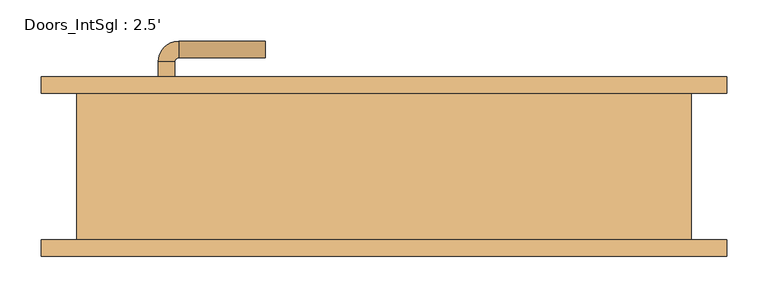
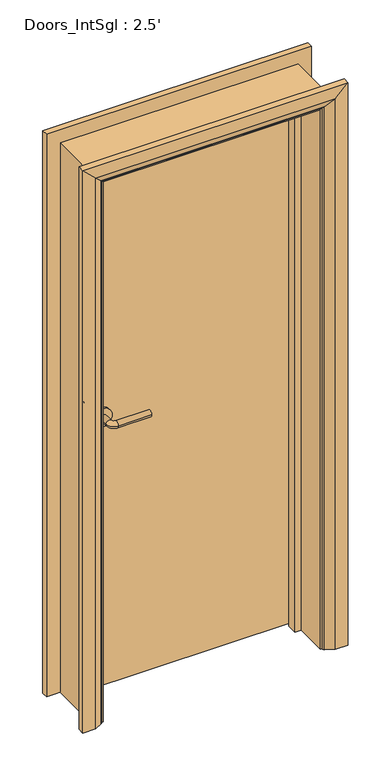
"""IFC4 building model written with IfcOpenShell, lengths in millimetres: door geometry, Doors_IntSgl : 2.5'."""

from ifc_helpers import new_model, si_unit, point, frame, frame_2d, origin, place, context, project, spatial, polyline, circle_curve, ellipse_curve, trimmed, segment, composite_curve, outline, extrude, faceted_brep, source, transform, mapped, element, save
from ifc_brep_helpers import plane_surface, cylinder_surface, revolved_surface, advanced_brep


def doors_intsgl_2_5_ea0f4f48(model_context):
    return source(origin(), model_context, "Body", "SolidModel", [
        advanced_brep(
        [(-274.0, 42.9, 900.0), (-254.0, 42.9, 900.0), (-254.0, 12.9, 900.0), (-274.0, 12.9, 900.0), (-249.0, 7.9, 900.0), (-249.0, -12.1, 900.0), (-144.0, -12.1, 900.0), (-144.0, 7.9, 900.0)],
        [
            (0, 1, circle_curve(frame((-264.0, 42.9, 900.0), z_axis=(0.0, 1.0, 0.0), x_axis=(1.0, 0.0, 0.0)), 10.0)),
            (1, 0, circle_curve(frame((-264.0, 42.9, 900.0), z_axis=(0.0, 1.0, 0.0), x_axis=(1.0, 0.0, 0.0)), 10.0)),
            (1, 2),
            (2, 3, circle_curve(frame((-264.0, 12.9, 900.0), z_axis=(0.0, 1.0, 0.0), x_axis=(1.0, 0.0, 0.0)), 10.0)),
            (3, 0),
            (3, 2, circle_curve(frame((-264.0, 12.9, 900.0), z_axis=(0.0, 1.0, 0.0), x_axis=(1.0, 0.0, 0.0)), 10.0)),
            (4, 5, circle_curve(frame((-249.0, -2.1, 900.0), z_axis=(-1.0, 0.0, 0.0), x_axis=(0.0, 1.0, 0.0)), 10.0)),
            (5, 3, circle_curve(frame((-249.0, 12.9, 900.0), z_axis=(0.0, 0.0, -1.0), x_axis=(-1.0, 0.0, 0.0)), 25.0)),
            (2, 4, circle_curve(frame((-249.0, 12.9, 900.0), z_axis=(0.0, 0.0, 1.0), x_axis=(-1.0, 0.0, 0.0)), 5.0)),
            (5, 4, circle_curve(frame((-249.0, -2.1, 900.0), z_axis=(-1.0, 0.0, 0.0), x_axis=(0.0, 1.0, 0.0)), 10.0)),
            (6, 7, circle_curve(frame((-144.0, -2.1, 900.0), z_axis=(1.0, 0.0, 0.0), x_axis=(0.0, 1.0, 0.0)), 10.0)),
            (7, 6, circle_curve(frame((-144.0, -2.1, 900.0), z_axis=(1.0, 0.0, 0.0), x_axis=(0.0, 1.0, 0.0)), 10.0)),
            (4, 7),
            (6, 5),
        ],
        [
            plane_surface(frame((-264.0, 42.9, 900.0), z_axis=(0.0, 1.0, 0.0), x_axis=(0.0, 0.0, 1.0))),
            cylinder_surface(frame((-264.0, 42.9, 900.0), z_axis=(0.0, 1.0, 0.0), x_axis=(1.0, 0.0, 0.0)), 10.0),
            revolved_surface(trimmed(ellipse_curve(frame((-264.0, 12.9, 900.0), z_axis=(0.0, -1.0, 0.0), x_axis=(1.0, 0.0, 0.0)), 10.0, 10.0), [point((-274.0, 12.9, 900.0))], [point((-254.0, 12.9, 900.0))], True, "CARTESIAN"), (-249.0, 12.9, 900.0), (0.0, 0.0, -1.0)),
            revolved_surface(trimmed(ellipse_curve(frame((-264.0, 12.9, 900.0), z_axis=(0.0, -1.0, 0.0), x_axis=(1.0, 0.0, 0.0)), 10.0, 10.0), [point((-254.0, 12.9, 900.0))], [point((-274.0, 12.9, 900.0))], True, "CARTESIAN"), (-249.0, 12.9, 900.0), (0.0, 0.0, -1.0)),
            plane_surface(frame((-144.0, -2.1, 900.0), z_axis=(1.0, 0.0, 0.0), x_axis=(0.0, 0.0, 1.0))),
            cylinder_surface(frame((-249.0, -2.1, 900.0), z_axis=(-1.0, 0.0, 0.0), x_axis=(0.0, 1.0, 0.0)), 10.0),
        ],
        [
            (0, [[1, 2]]),
            (1, [[3, 4, 5, -2]]),
            (1, [[-5, 6, -3, -1]]),
            (2, [[7, 8, -4, 9]]),
            (3, [[10, -9, -6, -8]]),
            (4, [[11, 12]]),
            (5, [[13, -11, 14, -7]]),
            (5, [[-14, -12, -13, -10]]),
        ],
    ),
        extrude(outline(composite_curve([segment(trimmed(circle_curve(frame_2d((900.0, -266.5)), 30.0), [point((900.0, -296.5))], [point((900.0, -236.5))], False, "CARTESIAN"), True, "CONTINUOUS"), segment(trimmed(circle_curve(frame_2d((900.0, -266.5)), 30.0), [point((900.0, -236.5))], [point((900.0, -296.5))], False, "CARTESIAN"), True, "CONTINUOUS")], self_intersect=False)), frame((0.0, 42.9, 0.0), z_axis=(0.0, 1.0, 0.0), x_axis=(0.0, 0.0, 1.0)), (0.0, 0.0, 1.0), 8.0),
        advanced_brep(
        [(-274.0, 96.9, 900.0), (-254.0, 96.9, 900.0), (-274.0, 126.9, 900.0), (-254.0, 126.9, 900.0), (-249.0, 131.9, 900.0), (-249.0, 151.9, 900.0), (-144.0, 151.9, 900.0), (-144.0, 131.9, 900.0)],
        [
            (0, 1, circle_curve(frame((-264.0, 96.9, 900.0), z_axis=(0.0, -1.0, 0.0), x_axis=(1.0, 0.0, 0.0)), 10.0)),
            (1, 0, circle_curve(frame((-264.0, 96.9, 900.0), z_axis=(0.0, -1.0, 0.0), x_axis=(1.0, 0.0, 0.0)), 10.0)),
            (0, 2),
            (2, 3, circle_curve(frame((-264.0, 126.9, 900.0), z_axis=(0.0, -1.0, 0.0), x_axis=(1.0, 0.0, 0.0)), 10.0)),
            (3, 1),
            (3, 2, circle_curve(frame((-264.0, 126.9, 900.0), z_axis=(0.0, -1.0, 0.0), x_axis=(1.0, 0.0, 0.0)), 10.0)),
            (4, 3, circle_curve(frame((-249.0, 126.9, 900.0), z_axis=(0.0, 0.0, 1.0), x_axis=(-1.0, 0.0, 0.0)), 5.0)),
            (2, 5, circle_curve(frame((-249.0, 126.9, 900.0), z_axis=(0.0, 0.0, -1.0), x_axis=(-1.0, 0.0, 0.0)), 25.0)),
            (5, 4, circle_curve(frame((-249.0, 141.9, 900.0), z_axis=(-1.0, 0.0, 0.0), x_axis=(0.0, -1.0, 0.0)), 10.0)),
            (4, 5, circle_curve(frame((-249.0, 141.9, 900.0), z_axis=(-1.0, 0.0, 0.0), x_axis=(0.0, -1.0, 0.0)), 10.0)),
            (6, 7, circle_curve(frame((-144.0, 141.9, 900.0), z_axis=(1.0, 0.0, 0.0), x_axis=(0.0, -1.0, 0.0)), 10.0)),
            (7, 6, circle_curve(frame((-144.0, 141.9, 900.0), z_axis=(1.0, 0.0, 0.0), x_axis=(0.0, -1.0, 0.0)), 10.0)),
            (5, 6),
            (7, 4),
        ],
        [
            plane_surface(frame((-264.0, 96.9, 900.0), z_axis=(0.0, -1.0, 0.0), x_axis=(0.0, 0.0, 1.0))),
            cylinder_surface(frame((-264.0, 96.9, 900.0), z_axis=(0.0, -1.0, 0.0), x_axis=(1.0, 0.0, 0.0)), 10.0),
            revolved_surface(trimmed(ellipse_curve(frame((-264.0, 126.9, 900.0), z_axis=(0.0, -1.0, 0.0), x_axis=(1.0, 0.0, 0.0)), 10.0, 10.0), [point((-274.0, 126.9, 900.0))], [point((-254.0, 126.9, 900.0))], True, "CARTESIAN"), (-249.0, 126.9, 900.0), (0.0, 0.0, -1.0)),
            revolved_surface(trimmed(ellipse_curve(frame((-264.0, 126.9, 900.0), z_axis=(0.0, -1.0, 0.0), x_axis=(1.0, 0.0, 0.0)), 10.0, 10.0), [point((-254.0, 126.9, 900.0))], [point((-274.0, 126.9, 900.0))], True, "CARTESIAN"), (-249.0, 126.9, 900.0), (0.0, 0.0, -1.0)),
            plane_surface(frame((-144.0, 141.9, 900.0), z_axis=(1.0, 0.0, 0.0), x_axis=(0.0, 0.0, 1.0))),
            cylinder_surface(frame((-249.0, 141.9, 900.0), z_axis=(-1.0, 0.0, 0.0), x_axis=(0.0, -1.0, 0.0)), 10.0),
        ],
        [
            (0, [[1, 2]]),
            (1, [[-1, 3, 4, 5]]),
            (1, [[-2, -5, 6, -3]]),
            (2, [[7, -4, 8, 9]]),
            (3, [[-8, -6, -7, 10]]),
            (4, [[11, 12]]),
            (5, [[-9, 13, -12, 14]]),
            (5, [[-10, -14, -11, -13]]),
        ],
    ),
        extrude(outline(composite_curve([segment(trimmed(circle_curve(frame_2d((900.0, -266.5)), 30.0), [point((900.0, -296.5))], [point((900.0, -236.5))], False, "CARTESIAN"), True, "CONTINUOUS"), segment(trimmed(circle_curve(frame_2d((900.0, -266.5)), 30.0), [point((900.0, -236.5))], [point((900.0, -296.5))], False, "CARTESIAN"), True, "CONTINUOUS")], self_intersect=False)), frame((0.0, 88.9, 0.0), z_axis=(0.0, 1.0, 0.0), x_axis=(0.0, 0.0, 1.0)), (0.0, 0.0, 1.0), 8.0),
        extrude(outline(polyline([(339.0, 50.9), (-339.0, 50.9), (-339.0, 88.9), (339.0, 88.9), (339.0, 50.9)])), frame((0.0, 0.0, 8.0), z_axis=(0.0, 0.0, 1.0), x_axis=(1.0, 0.0, 0.0)), (0.0, 0.0, 1.0), 1778.8),
        advanced_brep(
        [(416.0, 108.9, 0.0), (416.0, 88.9, 0.0), (346.0, 88.9, 0.0), (350.0, 94.9, 0.0), (376.0, 108.9, 0.0), (416.0, 108.9, 1863.8), (416.0, 88.9, 1863.8), (-416.0, 88.9, 1863.8), (-416.0, 88.9, 0.0), (-346.0, 88.9, 0.0), (-346.0, 88.9, 1793.8), (346.0, 88.9, 1793.8), (350.0, 94.9, 1797.8), (376.0, 108.9, 1823.8), (-376.0, 108.9, 1823.8), (-376.0, 108.9, 0.0), (-416.0, 108.9, 0.0), (-416.0, 108.9, 1863.8), (-350.0, 94.9, 0.0), (-350.0, 94.9, 1797.8)],
        [
            (0, 1),
            (1, 2),
            (2, 3, circle_curve(frame((354.0, 87.9, 0.0), z_axis=(0.0, 0.0, -1.0), x_axis=(1.0, 0.0, 0.0)), 8.0622577)),
            (3, 4),
            (4, 0),
            (0, 5),
            (5, 6),
            (6, 1),
            (6, 7),
            (7, 8),
            (8, 9),
            (9, 10),
            (10, 11),
            (11, 2),
            (11, 12, ellipse_curve(frame((354.0, 87.9, 1801.8), z_axis=(0.7071067811865475, 0.0, -0.7071067811865475), x_axis=(-0.7071067811865474, 0.0, -0.7071067811865476)), 11.4017543, 8.0622577)),
            (12, 3),
            (12, 13),
            (13, 4),
            (13, 14),
            (14, 15),
            (15, 16),
            (16, 17),
            (17, 5),
            (7, 17),
            (16, 8),
            (15, 18),
            (18, 9, circle_curve(frame((-354.0, 87.9, 0.0), z_axis=(0.0, 0.0, -1.0), x_axis=(-1.0, 0.0, 0.0)), 8.0622577)),
            (19, 10, ellipse_curve(frame((-354.0, 87.9, 1801.8), z_axis=(-0.7071067811865475, 0.0, -0.7071067811865475), x_axis=(-0.7071067811865474, 0.0, 0.7071067811865476)), 11.4017543, 8.0622577)),
            (18, 19),
            (14, 19),
            (19, 12),
        ],
        [
            plane_surface(frame((346.0, 88.9, 0.0), z_axis=(0.0, 0.0, -1.0), x_axis=(0.0, -1.0, 0.0))),
            plane_surface(frame((416.0, 108.9, 0.0), z_axis=(1.0, 0.0, 0.0), x_axis=(0.0, 0.0, 1.0))),
            plane_surface(frame((416.0, 88.9, 0.0), z_axis=(0.0, -1.0, 0.0), x_axis=(0.0, 0.0, 1.0))),
            cylinder_surface(frame((354.0, 87.9, 0.0), z_axis=(0.0, 0.0, -1.0), x_axis=(1.0, 0.0, 0.0)), 8.0622577),
            plane_surface(frame((350.0, 94.9, 0.0), z_axis=(-0.4740998230350126, 0.880471099922178, 0.0), x_axis=(0.0, 0.0, 1.0))),
            plane_surface(frame((376.0, 108.9, 0.0), z_axis=(0.0, 1.0, 0.0), x_axis=(0.0, 0.0, 1.0))),
            plane_surface(frame((-416.0, 108.9, 1863.8), z_axis=(-1.0, 0.0, 0.0), x_axis=(0.0, 0.0, -1.0))),
            plane_surface(frame((-346.0, 88.9, 0.0), z_axis=(0.0, 0.0, -1.0), x_axis=(0.0, -1.0, 0.0))),
            cylinder_surface(frame((-354.0, 87.9, 1793.8), z_axis=(0.0, 0.0, 1.0), x_axis=(-1.0, 0.0, 0.0)), 8.0622577),
            plane_surface(frame((-350.0, 94.9, 1797.8), z_axis=(0.47409982303501824, 0.8804710999221749, 0.0), x_axis=(0.0, 0.0, -1.0))),
            plane_surface(frame((416.0, 108.9, 1863.8), z_axis=(0.0, 0.0, 1.0), x_axis=(-1.0, 0.0, 0.0))),
            cylinder_surface(frame((346.0, 87.9, 1801.8), z_axis=(1.0, 0.0, 0.0), x_axis=(0.0, 0.0, 1.0)), 8.0622577),
            plane_surface(frame((350.0, 94.9, 1797.8), z_axis=(0.0, 0.8804710999221764, -0.4740998230350154), x_axis=(-1.0, 0.0, 0.0))),
        ],
        [
            (0, [[1, 2, 3, 4, 5]]),
            (1, [[-1, 6, 7, 8]]),
            (2, [[-2, -8, 9, 10, 11, 12, 13, 14]]),
            (3, [[-3, -14, 15, 16]]),
            (4, [[-4, -16, 17, 18]]),
            (5, [[-5, -18, 19, 20, 21, 22, 23, -6]]),
            (6, [[24, -22, 25, -10]]),
            (7, [[-21, 26, 27, -11, -25]]),
            (8, [[28, -12, -27, 29]]),
            (9, [[30, -29, -26, -20]]),
            (10, [[-7, -23, -24, -9]]),
            (11, [[-15, -13, -28, 31]]),
            (12, [[-17, -31, -30, -19]]),
        ],
    ),
        extrude(outline(polyline([(0.0, -341.0), (0.0, -322.0), (1769.8, -322.0), (1769.8, 322.0), (0.0, 322.0), (0.0, 341.0), (1788.8, 341.0), (1788.8, -341.0), (0.0, -341.0)])), frame((0.0, 16.9, 0.0), z_axis=(0.0, 1.0, 0.0), x_axis=(0.0, 0.0, 1.0)), (0.0, 0.0, 1.0), 32.0),
        advanced_brep(
        [(-416.0, -108.9, 0.0), (-416.0, -88.9, 0.0), (-346.0, -88.9, 0.0), (-350.0, -94.9, 0.0), (-376.0, -108.9, 0.0), (-416.0, -108.9, 1863.8), (-416.0, -88.9, 1863.8), (-346.0, -88.9, 1793.8), (-350.0, -94.9, 1797.8), (-376.0, -108.9, 1823.8), (416.0, -108.9, 0.0), (376.0, -108.9, 0.0), (350.0, -94.9, 0.0), (346.0, -88.9, 0.0), (416.0, -88.9, 0.0), (416.0, -108.9, 1863.8), (376.0, -108.9, 1823.8), (350.0, -94.9, 1797.8), (346.0, -88.9, 1793.8), (416.0, -88.9, 1863.8)],
        [
            (0, 1),
            (1, 2),
            (2, 3, circle_curve(frame((-354.0, -87.9, 0.0), z_axis=(0.0, 0.0, -1.0), x_axis=(-1.0, 0.0, 0.0)), 8.0622577)),
            (3, 4),
            (4, 0),
            (0, 5),
            (5, 6),
            (6, 1),
            (6, 7),
            (7, 2),
            (7, 8, ellipse_curve(frame((-354.0, -87.9, 1801.8), z_axis=(-0.7071067811865475, 0.0, -0.7071067811865475), x_axis=(0.7071067811865474, 0.0, -0.7071067811865476)), 11.4017543, 8.0622577)),
            (8, 3),
            (8, 9),
            (9, 4),
            (9, 5),
            (10, 11),
            (11, 12),
            (12, 13, circle_curve(frame((354.0, -87.9, 0.0), z_axis=(0.0, 0.0, -1.0), x_axis=(1.0, 0.0, 0.0)), 8.0622577)),
            (13, 14),
            (14, 10),
            (15, 16),
            (16, 11),
            (10, 15),
            (16, 17),
            (17, 12),
            (17, 18, ellipse_curve(frame((354.0, -87.9, 1801.8), z_axis=(0.7071067811865475, 0.0, -0.7071067811865475), x_axis=(0.7071067811865474, 0.0, 0.7071067811865476)), 11.4017543, 8.0622577)),
            (18, 13),
            (18, 19),
            (19, 14),
            (19, 15),
            (5, 15),
            (19, 6),
            (18, 7),
            (17, 8),
            (16, 9),
        ],
        [
            plane_surface(frame((-346.0, -161.7010989, 0.0), z_axis=(0.0, 0.0, -1.0), x_axis=(1.0, 0.0, 0.0))),
            plane_surface(frame((-416.0, -108.9, 0.0), z_axis=(-1.0, 0.0, 0.0), x_axis=(0.0, 0.0, 1.0))),
            plane_surface(frame((-416.0, -88.9, 0.0), z_axis=(0.0, 1.0, 0.0), x_axis=(0.0, 0.0, 1.0))),
            cylinder_surface(frame((-354.0, -87.9, 0.0), z_axis=(0.0, 0.0, -1.0), x_axis=(-1.0, 0.0, 0.0)), 8.0622577),
            plane_surface(frame((-350.0, -94.9, 0.0), z_axis=(0.4740998230350183, -0.8804710999221749, 0.0), x_axis=(0.0, 0.0, 1.0))),
            plane_surface(frame((-376.0, -108.9, 0.0), z_axis=(0.0, -1.0, 0.0), x_axis=(0.0, 0.0, 1.0))),
            plane_surface(frame((346.0, -161.7010989, 0.0), z_axis=(0.0, 0.0, -1.0), x_axis=(-1.0, 0.0, 0.0))),
            plane_surface(frame((376.0, -108.9, 1823.8), z_axis=(0.0, -1.0, 0.0), x_axis=(0.0, 0.0, -1.0))),
            plane_surface(frame((350.0, -94.9, 1797.8), z_axis=(-0.4740998230350183, -0.8804710999221749, 0.0), x_axis=(0.0, 0.0, -1.0))),
            cylinder_surface(frame((354.0, -87.9, 1793.8), z_axis=(0.0, 0.0, 1.0), x_axis=(1.0, 0.0, 0.0)), 8.0622577),
            plane_surface(frame((416.0, -88.9, 1863.8), z_axis=(0.0, 1.0, 0.0), x_axis=(0.0, 0.0, -1.0))),
            plane_surface(frame((416.0, -108.9, 1863.8), z_axis=(1.0, 0.0, 0.0), x_axis=(0.0, 0.0, -1.0))),
            plane_surface(frame((-416.0, -108.9, 1863.8), z_axis=(0.0, 0.0, 1.0), x_axis=(1.0, 0.0, 0.0))),
            plane_surface(frame((-416.0, -88.9, 1863.8), z_axis=(0.0, 1.0, 0.0), x_axis=(1.0, 0.0, 0.0))),
            cylinder_surface(frame((-346.0, -87.9, 1801.8), z_axis=(-1.0, 0.0, 0.0), x_axis=(0.0, 0.0, 1.0)), 8.0622577),
            plane_surface(frame((-350.0, -94.9, 1797.8), z_axis=(0.0, -0.8804710999221749, -0.4740998230350183), x_axis=(1.0, 0.0, 0.0))),
            plane_surface(frame((-376.0, -108.9, 1823.8), z_axis=(0.0, -1.0, 0.0), x_axis=(1.0, 0.0, 0.0))),
        ],
        [
            (0, [[1, 2, 3, 4, 5]]),
            (1, [[-1, 6, 7, 8]]),
            (2, [[-2, -8, 9, 10]]),
            (3, [[-3, -10, 11, 12]]),
            (4, [[-4, -12, 13, 14]]),
            (5, [[-5, -14, 15, -6]]),
            (6, [[16, 17, 18, 19, 20]]),
            (7, [[21, 22, -16, 23]]),
            (8, [[24, 25, -17, -22]]),
            (9, [[26, 27, -18, -25]]),
            (10, [[28, 29, -19, -27]]),
            (11, [[30, -23, -20, -29]]),
            (12, [[-7, 31, -30, 32]]),
            (13, [[-9, -32, -28, 33]]),
            (14, [[-11, -33, -26, 34]]),
            (15, [[-13, -34, -24, 35]]),
            (16, [[-15, -35, -21, -31]]),
        ],
    ),
        faceted_brep([(-341.0, 88.9, 0.0), (-341.0, -88.9, 0.0), (-373.0, -88.9, 0.0), (-373.0, 88.9, 0.0), (-341.0, 88.9, 1788.8), (-341.0, -88.9, 1788.8), (-373.0, -88.9, 1820.8), (-373.0, 88.9, 1820.8), (341.0, 88.9, 0.0), (373.0, 88.9, 0.0), (373.0, -88.9, 0.0), (341.0, -88.9, 0.0), (341.0, 88.9, 1788.8), (373.0, 88.9, 1820.8), (373.0, -88.9, 1820.8), (341.0, -88.9, 1788.8)], [[[0, 1, 2, 3]], [[1, 0, 4, 5]], [[2, 1, 5, 6]], [[3, 2, 6, 7]], [[0, 3, 7, 4]], [[8, 9, 10, 11]], [[12, 13, 9, 8]], [[13, 14, 10, 9]], [[14, 15, 11, 10]], [[15, 12, 8, 11]], [[5, 4, 12, 15]], [[6, 5, 15, 14]], [[7, 6, 14, 13]], [[4, 7, 13, 12]]]),
    ])


if __name__ == "__main__":
    model = new_model("IFC4")
    model_context = context("Model", 3, world=origin())
    ifc_project = project(units=[si_unit("LENGTHUNIT", "METRE", prefix="MILLI")], contexts=[model_context])
    site = spatial("IfcSite", under=ifc_project)
    building = spatial("IfcBuilding", under=site)
    placement = place(None, origin())
    doors_intsgl_2_5_shape = doors_intsgl_2_5_ea0f4f48(model_context)
    element("IfcDoor", 1, ObjectType="Doors_IntSgl : 2.5'", at=placement, inside=building, context=model_context, shape_type="MappedRepresentation", body=[
        mapped(doors_intsgl_2_5_shape, transform((0.0, 0.0, 0.0), x_axis=(1.0, 0.0, 0.0), y_axis=(0.0, 1.0, 0.0), z_axis=(0.0, 0.0, 1.0))),
    ])
    save(model, "model.ifc")

# Revit data of these elements
# Type "Doors_IntSgl : 2.5'"
#   Type Mark = "49"
#   Type Comments = "Internal Single"
#   Operation = "SingleSwingRight"
#   Manufacturer = "Revit"
#   Keynote = "L20"
#   Description = "Internal Single Door"
#   Analytic Construction = "Metal"
#   UnderCut = 0' - 0.31496"
#   Tolerance = 0' - 0.07874"
#   Thickness = 0' - 1.49606"
#   Thermal Resistance (R) = 0.270117 (m²·K)/W
#   Structural Tolerance = 0' - 0.31496"
#   StopDepth = 0' - 1.25984"
#   Stop Thickness = 0' - 0.74803"
#   Rough Width = 2' - 6"
#   Rough Height = 6' - 0"
#   Height to Top Lock Rail = 3' - 3.37008"
#   Heat Transfer Coefficient (U) = 3.7021 W/(m²·K)
#   Handle Z Distance = 2' - 11.43307"
#   Handle X Distance = 0' - 2.95276"
#   Frame Thickness = 0' - 1.25984"
#   Door Panel Width = 2' - 2.69291"
#   Door Panel Thickness = 0' - 1.49606"
#   Door Panel Offset = 0' - 0"
#   Height = 6' - 0"
#   Width = 2' - 6"
#   Door Panel Height = 5' - 10.0315"
#   Architrave Setback = 0' - 0.19685"
#   Vis - Ironmongery = yes
#   Material Ironmongery = Door - Handle
#   Material Frame = Door - Frame/Mullion (1)
#   Material Door = Door - Panel
#   Material Architrave = Door - Architrave
#   Visual Light Transmittance = 0
#   Solar Heat Gain Coefficient = 0
#   Function = (empty or 0)
#   Wall Closure = (empty or 0)
# Element 1 (IfcDoor, "Doors_IntSgl : 2.5'")
#   Materials on its faces: "Door - Architrave", "Door - Handle", "Door - Frame/Mullion (1)", "Door - Panel"
# Materials
#   "Door - Handle": colour RGB 0 0 0, transparency 0, Keynote = "P21", Cost = 0
#   "Door - Frame/Mullion (1)": class "Wood", colour RGB 212 179 113, transparency 0, Keynote = "L20", Cost = 0
#   "Door - Panel": class "Wood", colour RGB 210 159 95, transparency 0, Keynote = "L20", Cost = 0
#   "Door - Architrave": class "Wood", colour RGB 154 90 5, transparency 0, Keynote = "P20", Cost = 0
